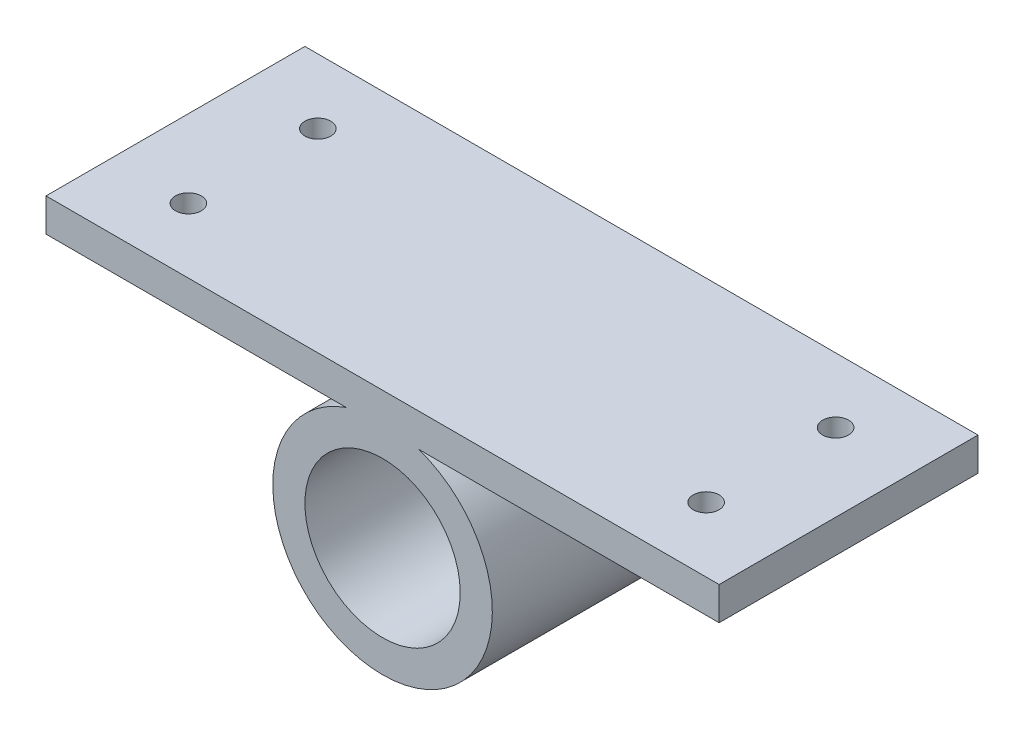
SolidWorks part; units mm, degrees
material "AISI 304"
ref_plane "Front Plane" through (0, 0, 0) normal (0, 0, 1) x (1, 0, 0)
ref_plane "Top Plane" through (0, 0, 0) normal (0, 1, 0) x (1, 0, 0)
ref_plane "Right Plane" through (0, 0, 0) normal (1, 0, 0) x (0, 0, -1)
sketch "Plate and Tube Profile Sketch" plane through (0, 0, 0) normal (0, 0, 1) x (1, 0, 0)
  line L0 (35.1568, -16) -> (325, -16)
  line L1 (-325, -16) -> (-35.1568, -16)
  line L2 (-325, -16) -> (-325, 16)
  line L3 (-325, 16) -> (325, 16)
  line L4 (325, -16) -> (325, 16)
  line L5 (-325, -16) -> (325, 16) construction
  line L6 (-325, 16) -> (325, -16) construction
  arc A0 (-35.1568, -16) -> (35.1568, -16) centre (0, -116) ccw
  circle A1 centre (0, -116) radius 75
  point P0 (0, 0)
  dimension "D4" = 212
  dimension "D5" = 150
  dimension "D1" = 32
  dimension "D2" = 650
  dimension "D3" = 132
extrude "Plate and Tube Body" add sketch "Plate and Tube Profile Sketch" along normal blind 250
sketch "Mounting Holes Sketch" plane through (0, 16, 0) normal (0, 1, 0) x (1, 0, 0)
  line L0 (-325, -250) -> (-325, 0) construction
  line L3 (325, 0) -> (-325, 0) construction
  line L4 (0, -130.9) -> (0, 130.9) construction
  circle A0 centre (-250, -62.5) radius 12.5
  circle A1 centre (250, -62.5) radius 12.5
  circle A2 centre (-250, -187.5) radius 12.5
  circle A3 centre (250, -187.5) radius 12.5
  dimension "D3" = 25
  dimension "D1" = 75
  dimension "D2" = 62.5
  dimension "D5" = 125
  dimension "D4" = 2
extrude "Mounting Holes 4x" cut sketch "Mounting Holes Sketch" against normal up to next
